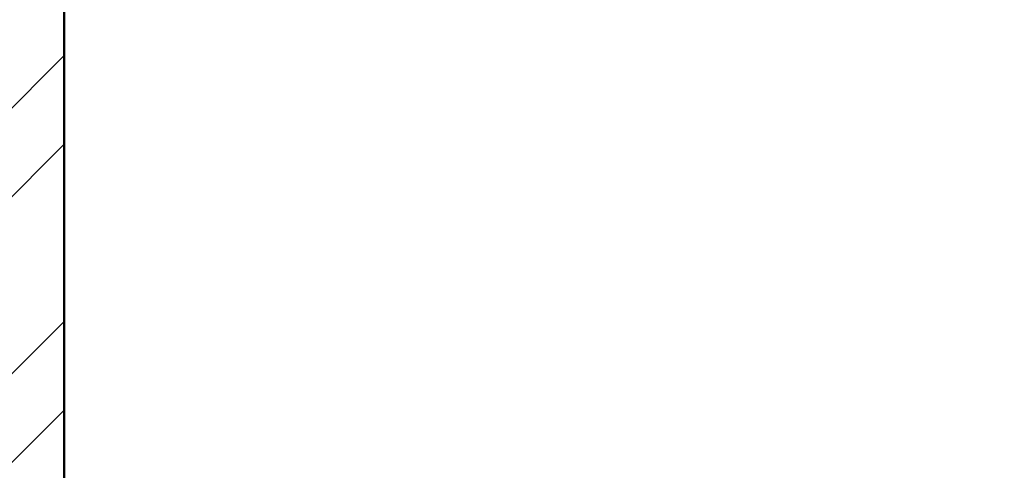
# Model space of a CAD drawing. Units: inches. Extents: x 963 to 2075, y 289 to 2657.
# Tile 7 of 98: x 1374 to 1424, y 1652 to 1675. Entities that reach past the tile are written whole.
import ezdxf

# ---------------------------------------------------------------- set-up
doc = ezdxf.new("R2010")
doc.units = ezdxf.units.IN
doc.layers.add('A-WALL', color=7, linetype='Continuous', lineweight=50)
doc.layers.add('A-WALL-PATT', color=8, linetype='Continuous', lineweight=13)

msp = doc.modelspace()

# ---------------------------------------------------------------- hatches: boundary and pattern name
at = {"layer": 'A-WALL-PATT'}
h = msp.add_hatch(dxfattribs=at)
h.set_pattern_fill('ANSI32', color=256)
h.paths.add_polyline_path([(1910.422, 1929.422), (1910.422, 1963.511), (1905.922, 1963.511), (1905.922, 1929.422), (1845.922, 1929.422), (1845.922, 1993.365), (1843.672, 1993.365), (1841.422, 1993.365), (1841.422, 1951.163), (1841.422, 1924.922), (1853.422, 1924.922), (1853.422, 1913.074), (1857.922, 1913.074), (1857.922, 1924.922), (1910.422, 1924.922)])
h.paths.add_polyline_path([(1857.922, 1853.074), (1853.422, 1853.074), (1853.422, 1826.318), (1841.422, 1826.318), (1674.482, 1826.318), (1674.482, 1821.818), (1853.422, 1821.818), (1857.922, 1821.818)])
h.paths.add_polyline_path([(1857.922, 1821.818), (1853.422, 1821.818), (1853.422, 1807.793), (1857.922, 1807.793)])
h.paths.add_polyline_path([(1857.922, 1747.793), (1853.422, 1747.793), (1853.422, 1713.818), (1809.343, 1713.818), (1809.343, 1709.318), (1905.922, 1709.318), (1905.922, 1688.318), (1910.422, 1688.318), (1910.422, 1713.818), (1857.922, 1713.818)])
h.paths.add_polyline_path([(1830.922, 1542.818), (1837.429, 1542.818), (1837.429, 1545.068), (1837.429, 1547.318), (1823.419, 1547.318), (1823.419, 1545.068), (1823.419, 1542.818), (1826.422, 1542.818), (1826.422, 1482.818), (1742.422, 1482.818), (1742.422, 1505.389), (1737.922, 1505.389), (1737.922, 1478.318), (1830.922, 1478.318)])
h.paths.add_polyline_path([(1938.922, 1619.318), (1934.422, 1619.318), (1910.422, 1619.318), (1910.422, 1628.318), (1908.172, 1628.318), (1905.922, 1628.318), (1905.922, 1614.818), (1934.422, 1614.818), (1934.422, 1547.318), (1905.922, 1547.318), (1899.589, 1547.318), (1899.589, 1542.818), (1910.422, 1542.818), (1938.922, 1542.818)])
h.paths.add_polyline_path([(1803.676, 1547.318), (1773.922, 1547.318), (1773.922, 1709.318), (1777.757, 1709.318), (1777.757, 1713.818), (1701.922, 1713.818), (1701.922, 1697.802), (1706.422, 1697.802), (1706.422, 1709.318), (1769.422, 1709.318), (1769.422, 1662.818), (1706.422, 1662.818), (1706.422, 1674.385), (1701.922, 1674.385), (1701.922, 1662.818), (1675.672, 1662.818), (1675.672, 1658.318), (1769.422, 1658.318), (1769.422, 1547.318), (1729.17, 1547.318), (1729.17, 1542.818), (1737.922, 1542.818), (1737.922, 1529.389), (1742.422, 1529.389), (1742.422, 1542.818), (1803.676, 1542.818)])
h.paths.add_polyline_path([(1595.422, 1542.818), (1599.245, 1542.818), (1599.245, 1547.318), (1584.36, 1547.318), (1584.36, 1542.818), (1590.922, 1542.818), (1590.922, 1436.318), (1595.422, 1436.318), (1595.422, 1440.818)])
h.paths.add_polyline_path([(1693.17, 1547.318), (1649.422, 1547.318), (1649.422, 1658.318), (1652.098, 1658.318), (1652.098, 1660.568), (1652.098, 1662.818), (1649.422, 1662.818), (1649.422, 1680.937), (1647.172, 1680.937), (1644.922, 1680.937), (1644.922, 1547.318), (1622.422, 1547.318), (1622.422, 1545.068), (1622.422, 1542.818), (1649.422, 1542.818), (1679.422, 1542.818), (1679.422, 1529.845), (1681.672, 1529.845), (1683.922, 1529.845), (1683.922, 1542.818), (1693.17, 1542.818), (1693.17, 1545.068)])
h.paths.add_polyline_path([(1683.922, 1505.845), (1679.422, 1505.845), (1679.422, 1483.805), (1595.422, 1483.805), (1595.422, 1479.305), (1683.922, 1479.305)])
h.paths.add_polyline_path([(1402.993, 1547.318), (1376.422, 1547.318), (1376.422, 1675.888), (1374.172, 1675.888), (1371.922, 1675.888), (1371.922, 1662.818), (1368.876, 1662.818), (1368.876, 1658.318), (1371.922, 1658.318), (1371.922, 1547.318), (1335.464, 1547.318), (1335.464, 1542.818), (1337.422, 1542.818), (1337.422, 1526.732), (1341.922, 1526.732), (1341.922, 1542.818), (1371.922, 1542.818), (1402.993, 1542.818)])

# ---------------------------------------------------------------- linework, layer by layer
at = {"layer": 'A-WALL'}
msp.add_line((1376.422, 1677.258), (1376.422, 1547.318), dxfattribs=at)

doc.saveas('drawing.dxf')
